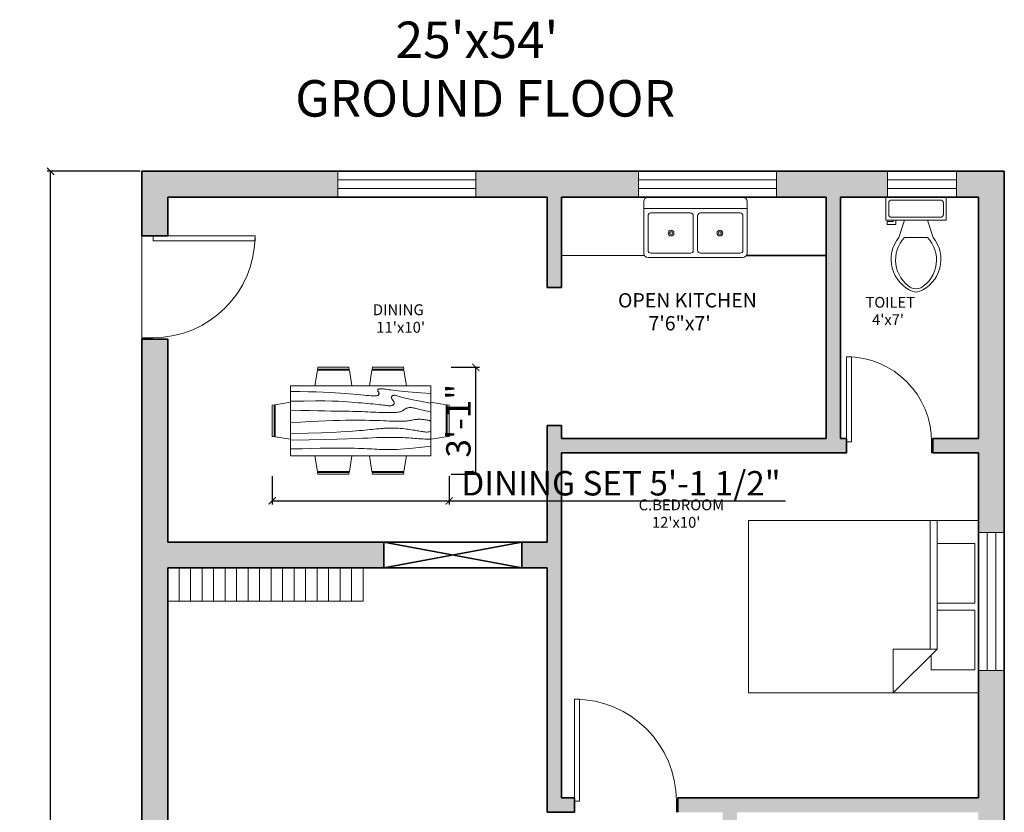
# Model space of a CAD drawing. Units: inches. Extents: x 3799 to 20199, y 1682 to 8087.
# Tile 27 of 30: x 16248 to 16590, y 7812 to 8087. Entities that reach past the tile are written whole.
import ezdxf

# ---------------------------------------------------------------- set-up
doc = ezdxf.new("R2010")
doc.units = ezdxf.units.IN
for name, color, linetype, lineweight in [('A-ANNO-DIMS', 2, 'Continuous', 18), ('A-ANNO-TITL', 7, 'Continuous', 25), ('A-AREA-IDEN', 7, 'Continuous', 18), ('A-DOOR', 3, 'Continuous', 18), ('A-FLOR-CASE', 32, 'Continuous', 18), ('A-FLOR-FIXT', 9, 'Continuous', 18), ('A-FURN', 8, 'Continuous', 18), ('A-GLAZ', 152, 'Continuous', 18), ('A-WALL', 7, 'Continuous', 35), ('A-WALL-PATT', 252, 'Continuous', 13)]:
    doc.layers.add(name, color=color, linetype=linetype, lineweight=lineweight)
doc.styles.get("Standard").update_dxf_attribs({"font": 'arial.ttf'})
doc.dimstyles.new('ISO-25', dxfattribs={"dimtxt": 8.5, "dimasz": 2.5, "dimexe": 1.25, "dimexo": 0.625, "dimtad": 1, "dimdec": 0, "dimlunit": 3, "dimtxsty": 'Standard', "dimblk": 'ARCHTICK', "dimcen": 2.5, "dimadec": 0, "dimazin": 0, "dimtfac": 1, "dimtdec": 0, "dimtmove": 0, "dimatfit": 3, "dimfxl": 1, "dimarcsym": 0})

# ---------------------------------------------------------------- blocks, each defined once
blk = doc.blocks.new('Dining Set - 36 x 72 in.')
for p, q in [((-22.2343, 26.00059), (-23.4847, 17.99762)), ((-22.2304, 26), (-5.7608, 26)), ((-22, 27.5), (-22.1562, 26.50042)), ((-5.8416, 26.5), (-22.1534, 26.5)), ((-22, 27.5), (-6, 27.5)), ((-5.8437, 26.49966), (-6, 27.5)), ((-4.5152, 17.99762), (-5.7655, 25.99926)), ((5.7657, 26.00059), (4.5153, 17.99762)), ((5.7696, 26), (22.2392, 26)), ((6, 27.5), (5.8438, 26.50042)), ((22.1584, 26.5), (5.8466, 26.5)), ((6, 27.5), (22, 27.5)), ((22.1563, 26.49966), (22, 27.5)), ((23.4848, 17.99762), (22.2345, 25.99926)), ((36, 18), (-36, 18)), ((-36, 18), (-36, -18)), ((36, -18), (36, 18)), ((-45.5, 8), (-44.5004, 8.15617)), ((-45.5, 8), (-45.5, -8)), ((-44.5, -8.15843), (-44.5, 8.15338)), ((-44.0006, 8.23428), (-35.9976, 9.48474)), ((-44, 8.23041), (-44, -8.23915)), ((44.0006, 8.23428), (35.9976, 9.48474)), ((44, 8.23041), (44, -8.23915)), ((44.5, -8.15843), (44.5, 8.15338)), ((45.5, 8), (44.5005, 8.15617)), ((45.5, 8), (45.5, -8)), ((-44.4997, -8.15631), (-45.5, -8)), ((-35.9976, -9.48476), (-43.9993, -8.2345)), ((35.9976, -9.48476), (43.9993, -8.2345)), ((44.4997, -8.15631), (45.5, -8)), ((-36, -18), (36, -18)), ((-22.2343, -26.0006), (-23.4847, -17.99762)), ((-4.5152, -17.99762), (-5.7655, -25.99928)), ((5.7657, -26.0006), (4.5153, -17.99762)), ((23.4848, -17.99762), (22.2345, -25.99928)), ((-22.2304, -26), (-5.7608, -26)), ((-22, -27.5), (-22.1562, -26.50044)), ((-5.8416, -26.5), (-22.1534, -26.5)), ((-22, -27.5), (-6, -27.5)), ((-5.8437, -26.49967), (-6, -27.5)), ((5.7696, -26), (22.2392, -26)), ((6, -27.5), (5.8438, -26.50044)), ((22.1584, -26.5), (5.8466, -26.5)), ((6, -27.5), (22, -27.5)), ((22.1563, -26.49967), (22, -27.5))]:
    blk.add_line(p, q)
for points in [[(-36, 15), (-31.1772, 14.97754), (-26.8079, 14.91406), (-22.8538, 14.81543), (-19.276, 14.6875), (-16.0362, 14.53613), (-13.0957, 14.36718), (-10.4159, 14.18652), (-7.9583, 14), (-5.6904, 13.81315), (-3.6035, 13.63021), (-1.6954, 13.45508), (0.0365, 13.29166), (1.5945, 13.14388), (2.9811, 13.01562), (4.1988, 12.9108), (5.25, 12.83333), (6.1393, 12.78613), (6.8802, 12.76823), (7.4883, 12.77767), (7.9792, 12.8125), (8.3685, 12.87077), (8.6719, 12.95052), (8.9049, 13.0498), (9.0833, 13.16666), (9.2205, 13.29899), (9.3216, 13.44401), (9.3895, 13.59879), (9.4271, 13.76041), (9.4373, 13.92594), (9.4232, 14.09245), (9.3875, 14.257), (9.3333, 14.41666), (9.2638, 14.56917), (9.1836, 14.71484), (9.0975, 14.85465), (9.0104, 14.98958), (8.9272, 15.1206), (8.8529, 15.2487), (8.7922, 15.37483), (8.75, 15.5), (8.7305, 15.62467), (8.7344, 15.74739), (8.7617, 15.86621), (8.8125, 15.97916), (8.8867, 16.08431), (8.9844, 16.17968), (9.1055, 16.26334), (9.25, 16.33333), (9.4189, 16.38802), (9.6172, 16.42708), (9.8506, 16.45052), (10.125, 16.45833), (10.4463, 16.45052), (10.8203, 16.42708), (11.2529, 16.38802), (11.75, 16.33333), (12.3184, 16.26318), (12.9694, 16.17838), (13.7151, 16.07991), (14.5677, 15.96875), (15.5395, 15.84586), (16.6426, 15.71224), (17.8893, 15.56884), (19.2917, 15.41666), (20.859, 15.25667), (22.5879, 15.08984), (24.4721, 14.91715), (26.5052, 14.73958), (28.6809, 14.5581), (30.9929, 14.3737), (33.4347, 14.18733), (36, 14)], [(-36, 10), (-28.9766, 10.14274), (-23.1725, 10.20442), (-18.4241, 10.19775), (-14.5677, 10.13541), (-11.4399, 10.03011), (-8.877, 9.89453), (-6.7154, 9.74137), (-4.7917, 9.58333), (-2.9698, 9.43082), (-1.2246, 9.28515), (0.4415, 9.14534), (2.026, 9.01041), (3.5266, 8.87939), (4.9408, 8.7513), (6.266, 8.62516), (7.5, 8.5), (8.6411, 8.37549), (9.6914, 8.2539), (10.6538, 8.13818), (11.5312, 8.03125), (12.3267, 7.93603), (13.043, 7.85547), (13.6831, 7.79248), (14.25, 7.75), (14.7471, 7.7303), (15.1797, 7.73307), (15.5537, 7.75732), (15.875, 7.80208), (16.1494, 7.86637), (16.3828, 7.94922), (16.5811, 8.04964), (16.75, 8.16666), (16.8944, 8.29915), (17.0143, 8.44531), (17.1089, 8.60319), (17.1771, 8.77083), (17.218, 8.94629), (17.2305, 9.1276), (17.2137, 9.31282), (17.1667, 9.5), (17.0895, 9.6875), (16.987, 9.875), (16.8649, 10.0625), (16.7292, 10.25), (16.5856, 10.4375), (16.4401, 10.625), (16.2985, 10.8125), (16.1667, 11), (16.05, 11.18733), (15.9518, 11.3737), (15.8752, 11.5581), (15.8229, 11.73958), (15.798, 11.91715), (15.8034, 12.08984), (15.842, 12.25667), (15.9167, 12.41666), (16.0295, 12.56836), (16.1784, 12.70833), (16.3605, 12.83268), (16.5729, 12.9375), (16.8127, 13.01888), (17.0768, 13.07291), (17.3625, 13.0957), (17.6667, 13.08333), (17.9894, 13.03312), (18.3418, 12.94726), (18.7382, 12.82918), (19.1927, 12.68229), (19.7195, 12.51001), (20.3327, 12.31575), (21.0465, 12.10294), (21.875, 11.875), (22.8357, 11.63354), (23.959, 11.37304), (25.2786, 11.08618), (26.8282, 10.76562), (28.6414, 10.40405), (30.752, 9.99414), (33.1936, 9.52856), (36, 9)], [(-36, 5.5), (-30.7157, 5.3348), (-26.069, 5.20963), (-21.9946, 5.11767), (-18.4271, 5.05208), (-15.3009, 5.00602), (-12.5508, 4.97265), (-10.1112, 4.94515), (-7.9167, 4.91666), (-5.909, 4.88167), (-4.0586, 4.83984), (-2.3429, 4.79215), (-0.7396, 4.73958), (0.7739, 4.6831), (2.22, 4.6237), (3.6213, 4.56233), (5, 4.5), (6.373, 4.43782), (7.7344, 4.3776), (9.0723, 4.32129), (10.375, 4.27083), (11.6309, 4.22819), (12.8281, 4.19531), (13.9551, 4.17415), (15, 4.16666), (15.954, 4.17448), (16.819, 4.19791), (17.6001, 4.23698), (18.3021, 4.29166), (18.9299, 4.36198), (19.4883, 4.44791), (19.9823, 4.54948), (20.4167, 4.66666), (20.7969, 4.79899), (21.1302, 4.94401), (21.4245, 5.09879), (21.6875, 5.26041), (21.9271, 5.42594), (22.1511, 5.59245), (22.3672, 5.757), (22.5834, 5.91666), (22.8065, 6.06868), (23.0404, 6.21093), (23.2879, 6.34147), (23.5521, 6.45833), (23.8358, 6.55957), (24.142, 6.64323), (24.4735, 6.70735), (24.8334, 6.75), (25.2235, 6.76969), (25.642, 6.76692), (26.0858, 6.74267), (26.5521, 6.69791), (27.0379, 6.63362), (27.5404, 6.55078), (28.0565, 6.45036), (28.5834, 6.33333), (29.1242, 6.19987), (29.7071, 6.04687), (30.3661, 5.87044), (31.1354, 5.66666), (32.0493, 5.43164), (33.142, 5.16146), (34.4475, 4.85221), (36, 4.5)], [(-36, -1), (-30.7915, -0.6591), (-26.0195, -0.38216), (-21.6519, -0.16284), (-17.6563, 0.00521), (-14.0005, 0.12833), (-10.6523, 0.21289), (-7.5796, 0.26522), (-4.75, 0.29166), (-2.134, 0.29793), (0.2878, 0.28711), (2.5317, 0.26163), (4.6146, 0.22396), (6.5529, 0.17651), (8.3633, 0.12174), (10.0623, 0.06209), (11.6667, 0), (13.1899, -0.06201), (14.6341, -0.1211), (15.9982, -0.17432), (17.2813, -0.21875), (18.4823, -0.25147), (19.6003, -0.26953), (20.6343, -0.27002), (21.5834, -0.25), (22.4481, -0.20768), (23.2357, -0.14584), (23.9549, -0.06836), (24.6146, 0.02083), (25.2235, 0.11784), (25.7904, 0.21875), (26.3241, 0.31966), (26.8334, 0.41666), (27.3265, 0.50618), (27.8099, 0.58593), (28.2894, 0.65397), (28.7709, 0.70833), (29.2601, 0.74707), (29.763, 0.76823), (30.2855, 0.76985), (30.8334, 0.75), (31.4088, 0.70784), (31.9994, 0.64713), (32.589, 0.57275), (33.1615, 0.48958), (33.7008, 0.4025), (34.1908, 0.3164), (34.6153, 0.23616), (34.9584, 0.16666), (35.2099, 0.11165), (35.3848, 0.07031), (35.504, 0.04069), (35.5886, 0.02083), (35.6594, 0.00879), (35.7377, 0.0026), (35.8442, 0.00032), (36, 0)], [(-36, -6.5), (-27.1843, -6.31267), (-20.084, -6.1263), (-14.469, -5.9419), (-10.1094, -5.76042), (-6.7752, -5.58285), (-4.2363, -5.41016), (-2.2629, -5.24333), (-0.625, -5.08334), (0.8708, -4.93099), (2.2715, -4.78646), (3.5872, -4.64974), (4.8281, -4.52084), (6.0046, -4.39974), (7.127, -4.28646), (8.2053, -4.18099), (9.25, -4.08334), (10.2705, -3.99382), (11.2734, -3.91407), (12.2647, -3.84603), (13.25, -3.79167), (14.2354, -3.75293), (15.2266, -3.73177), (16.2295, -3.73015), (17.25, -3.75), (18.2912, -3.79248), (19.3451, -3.85547), (20.4009, -3.93604), (21.4479, -4.03125), (22.4754, -4.13819), (23.4727, -4.25391), (24.4289, -4.37549), (25.3334, -4.5), (26.1785, -4.62492), (26.9694, -4.74935), (27.7145, -4.87281), (28.4219, -4.99479), (29.1, -5.11483), (29.7572, -5.23242), (30.4016, -5.34709), (31.0417, -5.45834), (31.6837, -5.56437), (32.3262, -5.65821), (32.9658, -5.73153), (33.599, -5.77604), (34.2224, -5.78345), (34.8327, -5.74545), (35.4264, -5.65373), (36, -5.5)], [(-36, -10), (-26.4022, -9.81299), (-18.4675, -9.62891), (-11.9839, -9.45069), (-6.7396, -9.28125), (-2.5226, -9.12354), (0.8789, -8.98047), (3.6769, -8.85498), (6.0833, -8.75), (8.2767, -8.66765), (10.3021, -8.60677), (12.1712, -8.56543), (13.8958, -8.54167), (15.4876, -8.53353), (16.9583, -8.53907), (18.3197, -8.55632), (19.5834, -8.58334), (20.7616, -8.61841), (21.8685, -8.66081), (22.9188, -8.71004), (23.9271, -8.76563), (24.9081, -8.82707), (25.8763, -8.89388), (26.8465, -8.96558), (27.8334, -9.04167), (28.8474, -9.12118), (29.8828, -9.20117), (30.93, -9.27824), (31.9792, -9.34896), (33.0205, -9.40991), (34.0443, -9.45768), (35.0407, -9.48885), (36, -9.5)], [(-36, -14.5), (-30.0881, -14.33513), (-25.0332, -14.21224), (-20.7312, -14.12647), (-17.0781, -14.07292), (-13.97, -14.04671), (-11.3027, -14.04297), (-8.9724, -14.05681), (-6.875, -14.08334), (-4.9224, -14.11833), (-3.0905, -14.16016), (-1.3709, -14.20785), (0.2448, -14.26042), (1.7647, -14.3169), (3.1973, -14.3763), (4.5507, -14.43767), (5.8333, -14.5), (7.0554, -14.5621), (8.235, -14.62175), (9.3922, -14.67652), (10.5469, -14.72396), (11.7192, -14.76164), (12.929, -14.78711), (14.1965, -14.79794), (15.5417, -14.79167), (16.9933, -14.76424), (18.6152, -14.70508), (20.4804, -14.60197), (22.6615, -14.44271), (25.2312, -14.21509), (28.2624, -13.9069), (31.8277, -13.50594), (36, -13)]]:
    blk.add_lwpolyline(points)
blk = doc.blocks.new('*U49')
for p, q in [((0, 0), (0, -100)), ((900, 0), (900, -100))]:
    blk.add_line(p, q)
blk.add_lwpolyline([(0, 0), (0, 900), (43.75, 900), (43.75, 0)], close=True)
blk.add_arc((0, 0), 900, 0, 90)
blk = doc.blocks.new('Sink-double - 36 in top')
for p, q in [((-18, -4), (18, -4)), ((-0.75, -18.5), (-0.75, -6.5)), ((0.75, -6.5), (0.75, -18.5))]:
    blk.add_line(p, q)
for points in [[(-16.5, 0), (16.5, 0)], [(-18, -19.5), (-18, -1.5)], [(18, -1.5), (18, -19.5)], [(-16.5, -18.5), (-16.5, -6.5)], [(-15.5, -5.5), (-1.75, -5.5)], [(1.75, -5.5), (15.5, -5.5)], [(16.5, -6.5), (16.5, -18.5)], [(-1.75, -19.5), (-15.5, -19.5)], [(15.5, -19.5), (1.75, -19.5)], [(16.5, -21), (-16.5, -21)]]:
    blk.add_lwpolyline(points)
for centre, radius in [((-8.5, -12.5), 1), ((-8.5, -12.5), 0.5), ((8.5, -12.5), 1), ((8.5, -12.5), 0.5)]:
    blk.add_circle(centre, radius)
for centre, radius, start, end in [((-16.5, -1.5), 1.5, 90, 180), ((16.5, -1.5), 1.5, 0, 90), ((-15.5, -6.5), 1, 90, 180), ((-1.75, -6.5), 1, 0, 90), ((1.75, -6.5), 1, 90, 180), ((15.5, -6.5), 1, 0, 90), ((-16.5, -19.5), 1.5, 180, 270), ((-15.5, -18.5), 1, 180, 270), ((-1.75, -18.5), 1, 270, 0), ((1.75, -18.5), 1, 180, 270), ((15.5, -18.5), 1, 270, 0), ((16.5, -19.5), 1.5, 270, 0)]:
    blk.add_arc(centre, radius, start, end)
blk = doc.blocks.new('Toilet - top')
for p, q in [((9.5, -6), (9.5, -2)), ((-10, -8.5), (-8, -8.5)), ((-10, -9.5), (-10, -8.5)), ((-7, -9.5), (-10, -9.5)), ((-8, -8.5), (-8, -8)), ((-7, -8), (-7, -9.5)), ((-4, -8), (-6, -14)), ((4, -8), (6, -14)), ((4, -14), (-4, -14))]:
    blk.add_line(p, q)
blk.add_lwpolyline([(10.5, -8), (10.5, 0), (-10.5, 0), (-10.5, -8)], close=True)
for points in [[(-9.5, -2), (-9.5, -6)], [(8.5, -1), (-8.5, -1)], [(-8.5, -7), (8.5, -7)]]:
    blk.add_lwpolyline(points)
for centre, radius, start, end in [((-8.62, -1.88), 0.884, 81.8699, 188.1301), ((8.62, -1.88), 0.884, 351.8699, 98.1301), ((-8.62, -6.12), 0.884, 171.8699, 278.1301), ((8.62, -6.12), 0.884, 261.8699, 8.1301), ((3.52, -21.58), 12.17, 141.4691, 247.9714), ((4.2, -21.82), 11.33, 136.3677, 238.9468), ((-3.52, -21.58), 12.17, 292.0284, 38.5307), ((-4.2, -21.82), 11.33, 301.053, 43.6321), ((0, -27.88), 4, 245.7318, 294.2682), ((0, -29), 4, 254.8605, 285.1395)]:
    blk.add_arc(centre, radius, start, end)
blk = doc.blocks.new('Bed - Queen')
for p, q in [((0, -80.00003), (0, 0)), ((0, 0), (59.99999, 0)), ((59.99999, 0), (59.99999, -80.00003)), ((7.99999, -1.2), (28.79998, -1.2)), ((7.99999, -14.4), (7.99999, -1.2)), ((28.79998, -1.2), (28.79998, -14.4)), ((31.19999, -1.2), (51.99999, -1.2)), ((31.19999, -14.4), (31.19999, -1.2)), ((51.99999, -1.2), (51.99999, -16.4)), ((0, -14.4), (44.8, -14.4)), ((44.8, -16.8), (0, -16.8)), ((59.99999, -29.6), (44.8, -14.4)), ((44.8, -14.4), (44.8, -29.6)), ((51.99999, -16.4), (46.79936, -16.4)), ((44.8, -29.6), (59.99999, -29.6)), ((59.99999, -80.00003), (0, -80.00003))]:
    blk.add_line(p, q)
blk = doc.blocks.new('*U47')
for p, q in [((0, 0), (0, -100)), ((750, 0), (750, -100))]:
    blk.add_line(p, q)
blk.add_lwpolyline([(0, 0), (0, 750), (43.75, 750), (43.75, 0)], close=True)
blk.add_arc((0, 0), 750, 0, 90)
blk = doc.blocks.new('WIN-24IN-9IN-FRAME')
for p, q in [((0, 24), (9, 24)), ((3, 0), (3, 24)), ((6, 0), (6, 24)), ((0, 0), (9, 0))]:
    blk.add_line(p, q)
blk = doc.blocks.new('WIN-48IN-9IN-FRAME')
for p, q in [((0, 0), (0, 9)), ((48, 0), (48, 9)), ((48, 6), (0, 6)), ((48, 3), (0, 3))]:
    blk.add_line(p, q)
blk = doc.blocks.new('_ArchTick')
at = {"color": 0, "linetype": 'ByBlock', "const_width": 0.15}
blk.add_lwpolyline([(-0.5, -0.5), (0.5, 0.5)], dxfattribs=at)
blk = doc.blocks.new('*D294')
at = {"layer": 'A-ANNO-DIMS', "color": 0, "lineweight": -2, "transparency": 16777216}
for p, q in [((16335.64, 7928.62), (16335.64, 7918.75)), ((16397.25, 7928.62), (16397.25, 7918.75)), ((16335.64, 7920), (16397.25, 7920)), ((16397.25, 7920), (16514.23, 7920))]:
    blk.add_line(p, q, dxfattribs=at)
at = {"layer": 'Defpoints', "color": 0, "transparency": 16777216}
for p in [(16335.64, 7929.24), (16397.25, 7929.24), (16397.25, 7920)]:
    blk.add_point(p, dxfattribs=at)
at = {"layer": 'A-ANNO-DIMS', "color": 0, "lineweight": -2, "transparency": 16777216, "xscale": 2.5, "yscale": 2.5, "zscale": 2.5, "rotation": 180}
blk.add_blockref('_ArchTick', (16335.64, 7920), dxfattribs=at)
at = {"layer": 'A-ANNO-DIMS', "color": 0, "lineweight": -2, "transparency": 16777216, "xscale": 2.5, "yscale": 2.5, "zscale": 2.5}
blk.add_blockref('_ArchTick', (16397.25, 7920), dxfattribs=at)
at = {"layer": 'A-ANNO-DIMS', "color": 0, "transparency": 16777216, "insert": (16456.99, 7925.02), "char_height": 8.5, "attachment_point": 5}
blk.add_mtext('DINING SET 5\'-1 1/2"', dxfattribs=at)
blk = doc.blocks.new('*D295')
at = {"layer": 'A-ANNO-DIMS', "color": 0, "lineweight": -2, "transparency": 16777216}
for p, q in [((16397.88, 7966.48), (16407.74, 7966.48)), ((16406.49, 7929.24), (16406.49, 7966.48)), ((16397.88, 7929.24), (16407.74, 7929.24))]:
    blk.add_line(p, q, dxfattribs=at)
at = {"layer": 'Defpoints', "color": 0, "transparency": 16777216}
for p in [(16397.25, 7966.48), (16406.49, 7966.48), (16397.25, 7929.24)]:
    blk.add_point(p, dxfattribs=at)
at = {"layer": 'A-ANNO-DIMS', "color": 0, "lineweight": -2, "transparency": 16777216, "xscale": 2.5, "yscale": 2.5, "zscale": 2.5}
for p, rotation in [((16406.49, 7966.48), 90), ((16406.49, 7929.24), 270)]:
    blk.add_blockref('_ArchTick', p, dxfattribs=dict(at, rotation=rotation))
at = {"layer": 'A-ANNO-DIMS', "color": 0, "transparency": 16777216, "insert": (16401.53, 7947.86), "char_height": 8.5, "attachment_point": 5, "rotation": 90}
blk.add_mtext('3\'-1"', dxfattribs=at)
blk = doc.blocks.new('*D359')
at = {"layer": 'A-ANNO-DIMS', "color": 0, "lineweight": -2, "transparency": 16777216}
for p, q in [((16289.71, 8034.65), (16257.33, 8034.65)), ((16258.58, 7494.65), (16258.58, 8034.65)), ((16289.71, 7494.65), (16257.33, 7494.65))]:
    blk.add_line(p, q, dxfattribs=at)
at = {"layer": 'Defpoints', "color": 0, "transparency": 16777216}
for p in [(16258.58, 8034.65), (16290.33, 8034.65), (16290.33, 7494.65)]:
    blk.add_point(p, dxfattribs=at)
at = {"layer": 'A-ANNO-DIMS', "color": 0, "lineweight": -2, "transparency": 16777216, "xscale": 2.5, "yscale": 2.5, "zscale": 2.5}
for p, rotation in [((16258.58, 8034.65), 90), ((16258.58, 7494.65), 270)]:
    blk.add_blockref('_ArchTick', p, dxfattribs=dict(at, rotation=rotation))
at = {"layer": 'A-ANNO-DIMS', "color": 0, "transparency": 16777216, "insert": (16253.62, 7764.65), "char_height": 8.5, "attachment_point": 5, "rotation": 90}
blk.add_mtext('45\'-0"', dxfattribs=at)

msp = doc.modelspace()

# ---------------------------------------------------------------- hatches: boundary and pattern name
at = {"layer": 'A-WALL-PATT'}
h = msp.add_hatch(color=256, dxfattribs=at)
h.dxf.hatch_style = 1
h.paths.add_polyline_path([(16358.47, 8034.65), (16290.33, 8034.65), (16290.33, 8012.2), (16294.27, 8012.2), (16299.33, 8012.2), (16299.33, 8025.65), (16358.47, 8025.65)])
h.paths.add_polyline_path([(16463.1, 8034.65), (16406.47, 8034.65), (16406.47, 8025.65), (16431.33, 8025.65), (16431.33, 7994.23), (16436.33, 7994.23), (16436.33, 8025.65), (16463.1, 8025.65)])
h.paths.add_polyline_path([(16549.72, 8034.65), (16511.1, 8034.65), (16511.1, 8025.65), (16528.33, 8025.65), (16528.33, 7941.65), (16436.33, 7941.65), (16436.33, 7946.23), (16431.33, 7946.23), (16431.33, 7905.65), (16422.55, 7905.65), (16422.55, 7896.65), (16431.33, 7896.65), (16431.33, 7811.65), (16440.82, 7811.65), (16440.82, 7816.65), (16436.33, 7816.65), (16436.33, 7936.65), (16533.33, 7936.65), (16535.49, 7936.65), (16535.49, 7941.65), (16533.33, 7941.65), (16533.33, 8025.65), (16549.72, 8025.65)])
h.paths.add_polyline_path([(16590.33, 8034.65), (16573.72, 8034.65), (16573.72, 8025.65), (16581.33, 8025.65), (16581.33, 7941.65), (16565.49, 7941.65), (16565.49, 7936.65), (16581.33, 7936.65), (16581.33, 7908.97), (16590.33, 7908.97)])
h.paths.add_polyline_path([(16590.33, 7860.97), (16581.33, 7860.97), (16581.33, 7853.17), (16581.33, 7816.65), (16476.82, 7816.65), (16476.82, 7811.65), (16492.33, 7811.65), (16492.33, 7763.65), (16476.82, 7763.65), (16476.82, 7758.65), (16498.62, 7758.65), (16498.62, 7762.58), (16498.62, 7763.65), (16497.33, 7763.65), (16497.33, 7811.65), (16581.33, 7811.65), (16581.33, 7797.89), (16590.33, 7797.89)])
h.paths.add_polyline_path([(16590.33, 7773.89), (16581.33, 7773.89), (16581.33, 7763.65), (16528.62, 7763.65), (16528.62, 7758.65), (16581.33, 7758.65), (16581.33, 7725.04), (16590.33, 7725.04)])
h.paths.add_polyline_path([(16590.33, 7677.04), (16581.33, 7677.04), (16581.33, 7665.04), (16581.33, 7626.65), (16581.33, 7503.65), (16427.6, 7503.65), (16427.6, 7494.65), (16590.33, 7494.65)])
h.paths.add_polyline_path([(16581.33, 7626.65), (16436.33, 7626.65), (16436.33, 7758.65), (16440.82, 7758.65), (16440.82, 7759.71), (16440.82, 7763.65), (16431.33, 7763.65), (16431.33, 7646.65), (16418.83, 7646.65), (16418.83, 7637.65), (16431.33, 7637.65), (16431.33, 7617.65), (16581.33, 7617.65)])
h.paths.add_polyline_path([(16309.09, 7646.65), (16299.33, 7646.65), (16299.33, 7702.3), (16290.33, 7702.3), (16290.33, 7494.65), (16304.67, 7494.65), (16304.67, 7503.65), (16299.33, 7503.65), (16299.33, 7637.65), (16309.09, 7637.65), (16309.09, 7641.58)])
h.paths.add_polyline_path([(16299.33, 7896.65), (16374.55, 7896.65), (16374.55, 7905.65), (16299.33, 7905.65), (16299.33, 7976.2), (16290.33, 7976.2), (16290.33, 7750.3), (16299.33, 7750.3)])
h.paths.add_polyline_path([(16370.83, 7646.65), (16345.09, 7646.65), (16345.09, 7637.65), (16370.83, 7637.65)])

# ---------------------------------------------------------------- linework, layer by layer
at = {"layer": 'A-DOOR'}
msp.add_line((16290.33, 8012.2), (16290.33, 7976.2), dxfattribs=at)
at = {"layer": 'A-FLOR-CASE'}
for p, q in [((16436.33, 8005.33), (16465.14, 8005.33)), ((16303.29, 7896.65), (16303.29, 7885.05)), ((16307.29, 7896.65), (16307.29, 7885.05)), ((16311.29, 7896.65), (16311.29, 7885.05)), ((16315.29, 7896.65), (16315.29, 7885.05)), ((16319.29, 7896.65), (16319.29, 7885.05)), ((16323.29, 7896.65), (16323.29, 7885.05)), ((16327.29, 7896.65), (16327.29, 7885.05)), ((16331.29, 7896.65), (16331.29, 7885.05)), ((16335.29, 7896.65), (16335.29, 7885.05)), ((16339.29, 7896.65), (16339.29, 7885.05)), ((16343.29, 7896.65), (16343.29, 7885.05)), ((16347.29, 7896.65), (16347.29, 7885.05)), ((16351.29, 7896.65), (16351.29, 7885.05)), ((16355.29, 7896.65), (16355.29, 7885.05)), ((16359.29, 7896.65), (16359.29, 7885.05)), ((16363.29, 7896.65), (16363.29, 7885.05)), ((16367.29, 7896.65), (16367.29, 7885.05)), ((16367.29, 7885.05), (16299.33, 7885.05))]:
    msp.add_line(p, q, dxfattribs=at)
at = {"layer": 'A-WALL'}
for p, q in [((16590.33, 8034.65), (16290.33, 8034.65)), ((16290.33, 8034.65), (16290.33, 8012.2)), ((16590.33, 7494.65), (16590.33, 8034.65)), ((16299.33, 8025.65), (16299.33, 8012.2)), ((16431.33, 8025.65), (16299.33, 8025.65)), ((16431.33, 8025.65), (16431.33, 7994.23)), ((16436.33, 8025.65), (16436.33, 7994.23)), ((16528.33, 8025.65), (16436.33, 8025.65)), ((16528.33, 7941.65), (16528.33, 8025.65)), ((16581.33, 8025.65), (16533.33, 8025.65)), ((16533.33, 7941.65), (16533.33, 8025.65)), ((16581.33, 7941.65), (16581.33, 8025.65)), ((16299.33, 8012.2), (16290.33, 8012.2)), ((16500.66, 8005.33), (16528.33, 8005.33)), ((16436.33, 7994.23), (16431.33, 7994.23)), ((16299.33, 7976.2), (16290.33, 7976.2)), ((16290.33, 7976.2), (16290.33, 7494.65)), ((16299.33, 7976.2), (16299.33, 7905.65)), ((16436.33, 7946.23), (16431.33, 7946.23)), ((16431.33, 7946.23), (16431.33, 7905.65)), ((16436.33, 7946.23), (16436.33, 7941.65)), ((16528.33, 7941.65), (16436.33, 7941.65)), ((16535.49, 7941.65), (16533.33, 7941.65)), ((16535.49, 7941.65), (16535.49, 7936.65)), ((16581.33, 7941.65), (16565.49, 7941.65)), ((16565.49, 7941.65), (16565.49, 7936.65)), ((16436.33, 7936.65), (16436.33, 7816.65)), ((16533.33, 7936.65), (16436.33, 7936.65)), ((16535.49, 7936.65), (16533.33, 7936.65)), ((16581.33, 7936.65), (16565.49, 7936.65)), ((16581.33, 7816.65), (16581.33, 7936.65)), ((16431.33, 7905.65), (16299.33, 7905.65)), ((16374.55, 7905.65), (16374.55, 7896.65)), ((16374.55, 7905.65), (16422.55, 7896.65)), ((16422.55, 7905.65), (16374.55, 7896.65)), ((16422.55, 7905.65), (16422.55, 7896.65)), ((16431.33, 7896.65), (16299.33, 7896.65)), ((16299.33, 7896.65), (16299.33, 7646.65)), ((16431.33, 7896.65), (16431.33, 7811.65)), ((16440.82, 7816.65), (16436.33, 7816.65)), ((16440.82, 7816.65), (16440.82, 7811.65)), ((16581.33, 7816.65), (16476.82, 7816.65)), ((16476.82, 7816.65), (16476.82, 7811.65)), ((16440.82, 7811.65), (16431.33, 7811.65))]:
    msp.add_line(p, q, dxfattribs=at)

# ---------------------------------------------------------------- block references
at = {"layer": 'A-DOOR', "xscale": 0.0393700787401575, "yscale": 0.0393700787401575, "zscale": 0.0393700787401575, "rotation": 270}
msp.add_blockref('*U49', (16294.27, 8012.2), dxfattribs=at)
at = {"layer": 'A-DOOR', "xscale": 0.0393700787401575, "yscale": 0.0393700787401575, "zscale": 0.0393700787401575}
for name, p in [('*U47', (16535.49, 7940.58)), ('*U49', (16440.82, 7815.58))]:
    msp.add_blockref(name, p, dxfattribs=at)
at = {"layer": 'A-FLOR-FIXT'}
for name, p in [('Sink-double - 36 in top', (16482.9, 8025.65)), ('Toilet - top', (16559.63, 8025.65))]:
    msp.add_blockref(name, p, dxfattribs=at)
at = {"layer": 'A-FURN', "xscale": 0.6771113843329873, "yscale": 0.6771113843329873, "zscale": 0.6771113843329873}
msp.add_blockref('Dining Set - 36 x 72 in.', (16366.44, 7947.86), dxfattribs=at)
at = {"layer": 'A-FURN', "rotation": 270}
msp.add_blockref('Bed - Queen', (16581.33, 7913.17), dxfattribs=at)
at = {"layer": 'A-GLAZ'}
for p in [(16358.47, 8025.65), (16463.1, 8025.65)]:
    msp.add_blockref('WIN-48IN-9IN-FRAME', p, dxfattribs=at)
at = {"layer": 'A-GLAZ', "rotation": 90}
for name, p in [('WIN-24IN-9IN-FRAME', (16573.72, 8025.65)), ('WIN-48IN-9IN-FRAME', (16590.33, 7860.97))]:
    msp.add_blockref(name, p, dxfattribs=at)

# ---------------------------------------------------------------- texts
at = {"layer": 'A-ANNO-TITL'}
for s, p in [("         25'x54'", (16343.69, 8074.05)), ('GROUND FLOOR', (16343.69, 8053.68))]:
    msp.add_text(s, height=12.6834, rotation=0.0017, dxfattribs=at).set_placement(p)
at = {"layer": 'A-AREA-IDEN'}
for s, height, p in [('OPEN KITCHEN', 4.9664, (16455.95, 7987.29)), ('TOILET', 3.747, (16542.07, 7987.2)), ('DINING', 3.807, (16370.67, 7984.58)), ('       7\'6"x7\'', 4.9664, (16455.95, 7979.31)), ("  4'x7'", 3.747, (16542.07, 7981.18)), (" 11'x10'", 3.807, (16370.67, 7978.47)), ('C.BEDROOM', 3.775, (16463.14, 7916.71)), ("    12'x10'", 3.7751, (16463.14, 7910.64))]:
    msp.add_text(s, height=height, rotation=0.0017, dxfattribs=at).set_placement(p)

# ---------------------------------------------------------------- dimensions: what is measured, and where the dimension line sits
at = {"layer": 'A-ANNO-DIMS'}
for base, p1, p2, picture, middle in [((16258.58, 8034.65), (16290.33, 7494.65), (16290.33, 8034.65), '*D359', (16253.62, 7764.65)), ((16406.49, 7966.48), (16397.25, 7929.24), (16397.25, 7966.48), '*D295', (16401.53, 7947.86))]:
    dim = msp.add_linear_dim(base=base, p1=p1, p2=p2, angle=90, dimstyle='ISO-25', override={"dimdec": 1, "dimlfac": 1, "dimrnd": 0, "dimzin": 1, "dimdsep": 46, "dimlunit": 4, "dimfrac": 2}, dxfattribs=at)
    dim.commit()
    dim.dimension.update_dxf_attribs({"geometry": picture, "text_midpoint": middle})
dim = msp.add_linear_dim(base=(16397.25, 7920), p1=(16335.64, 7929.24), p2=(16397.25, 7929.24), text='DINING SET <>', dimstyle='ISO-25', override={"dimdec": 1, "dimlfac": 1, "dimrnd": 0, "dimzin": 1, "dimdsep": 46, "dimlunit": 4, "dimfrac": 2}, dxfattribs=at)
dim.commit()
dim.dimension.update_dxf_attribs({"geometry": '*D294', "text_midpoint": (16456.99, 7925.02)})

doc.saveas('drawing.dxf')
